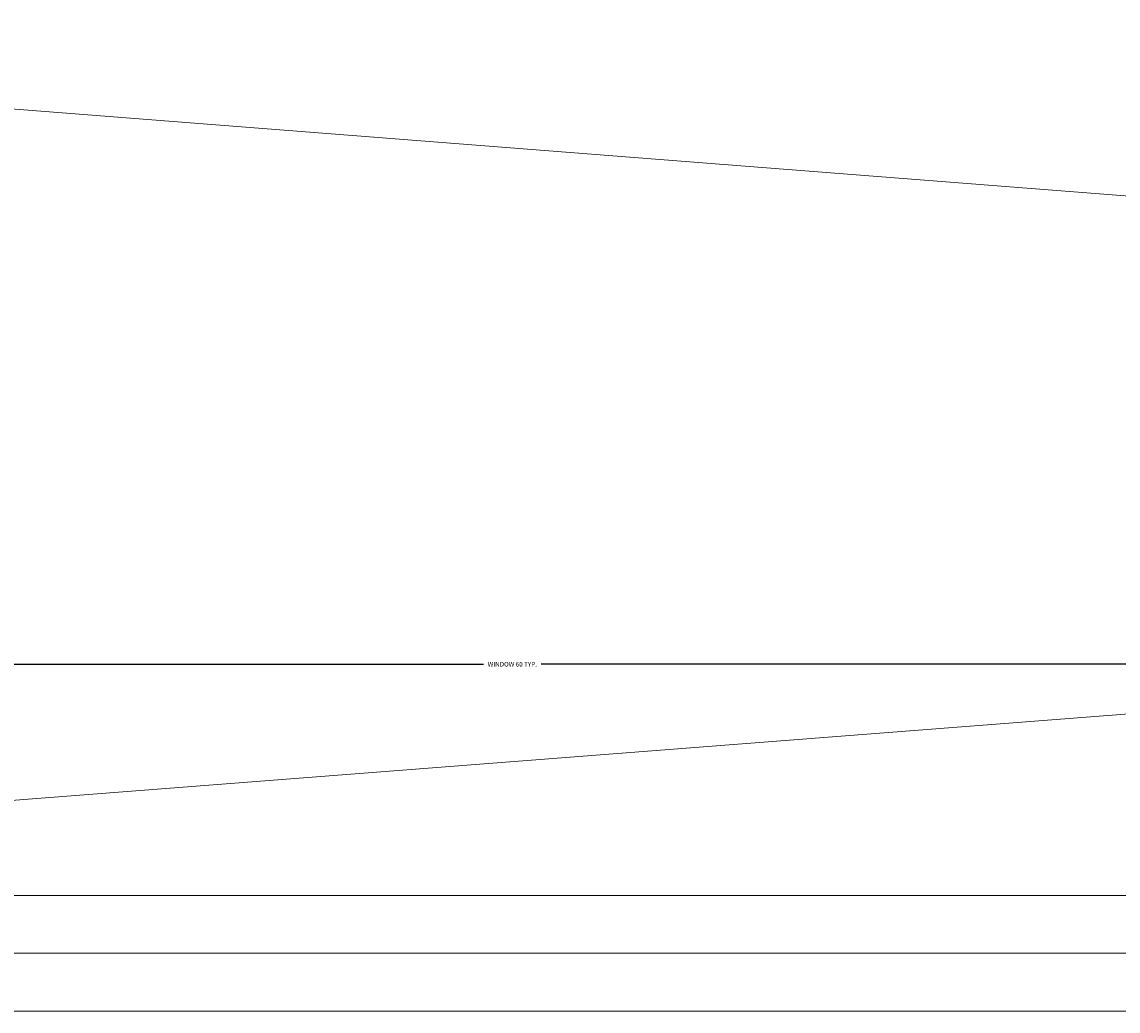
# Model space of a CAD drawing. Units: inches. Extents: x 1885 to 2748, y 783 to 2421.
# Tile 39 of 117: x 2056 to 2098, y 1520 to 1558. Entities that reach past the tile are written whole.
import ezdxf

# ---------------------------------------------------------------- set-up
doc = ezdxf.new("R2010")
doc.units = ezdxf.units.IN
for name, color, linetype, lineweight in [('A-ANNO-DIMS', 2, 'Continuous', 18), ('A-FLOR-OPEN', 8, 'Continuous', 13), ('A-GLAZ', 181, 'Continuous', 18)]:
    doc.layers.add(name, color=color, linetype=linetype, lineweight=lineweight)
doc.styles.get("Standard").update_dxf_attribs({"font": 'arial.ttf'})
doc.dimstyles.get("Standard").update_dxf_attribs({"dimtxt": 0.18, "dimasz": 0.18, "dimexe": 0.18, "dimexo": 0.0625, "dimgap": 0.09, "dimtad": 0, "dimtih": 1, "dimtoh": 1, "dimdec": 4, "dimzin": 0, "dimdsep": 46, "dimtxsty": 'Standard', "dimcen": 0.09, "dimadec": 0, "dimazin": 0, "dimtfac": 1, "dimtdec": 4, "dimtofl": 0, "dimtmove": 0, "dimatfit": 3, "dimfxl": 1, "dimtolj": 1, "dimtzin": 0, "dimarcsym": 0})

# ---------------------------------------------------------------- blocks, each defined once
blk = doc.blocks.new('WIN-60')
for p, q in [((0.004, 59.998), (4.504, 59.998)), ((0.004, 59.998), (0.004, -0.002)), ((4.504, 59.998), (2.254, 59.998)), ((2.254, 59.998), (2.254, -0.002)), ((4.504, -0.002), (4.504, 59.998)), ((2.254, -0.002), (0.004, -0.002)), ((0.004, -0.002), (4.504, -0.002))]:
    blk.add_line(p, q)
blk = doc.blocks.new('*D15')
at = {"layer": 'A-ANNO-DIMS', "color": 0, "lineweight": -2, "transparency": 16777216}
for p, q in [((2044.674, 1524.068), (2044.674, 1533.186)), ((2104.674, 1524.068), (2104.674, 1533.186)), ((2044.854, 1533.006), (2073.556, 1533.006)), ((2104.494, 1533.006), (2075.793, 1533.006))]:
    blk.add_line(p, q, dxfattribs=at)
at = {"layer": 'A-ANNO-DIMS', "color": 0, "transparency": 16777216}
for points in [[(2044.854, 1533.036), (2044.854, 1532.976), (2044.674, 1533.006)], [(2104.494, 1533.036), (2104.494, 1532.976), (2104.674, 1533.006)]]:
    blk.add_solid(points, dxfattribs=at)
at = {"layer": 'Defpoints', "color": 0, "transparency": 16777216}
for p in [(2104.674, 1533.006), (2044.674, 1524.006), (2104.674, 1524.006)]:
    blk.add_point(p, dxfattribs=at)
at = {"layer": 'A-ANNO-DIMS', "color": 0, "transparency": 16777216, "insert": (2074.674, 1533.006), "char_height": 0.18, "attachment_point": 5}
blk.add_mtext('\\A1;WINDOW 60 TYP.', dxfattribs=at)

msp = doc.modelspace()

# ---------------------------------------------------------------- linework, layer by layer
at = {"layer": 'A-FLOR-OPEN'}
for p, q in [((2007.274, 1524.006), (2447.274, 1558.006)), ((2447.274, 1524.006), (2011.774, 1558.006))]:
    msp.add_line(p, q, dxfattribs=at)

# ---------------------------------------------------------------- block references
at = {"layer": 'A-GLAZ', "extrusion": (0, 0, -1), "zscale": -1, "rotation": 90}
msp.add_blockref('WIN-60', (-2044.676, 1519.502), dxfattribs=at)

# ---------------------------------------------------------------- dimensions: what is measured, and where the dimension line sits
at = {"layer": 'A-ANNO-DIMS'}
dim = msp.add_linear_dim(base=(2104.674, 1533.006), p1=(2044.674, 1524.006), p2=(2104.674, 1524.006), text='WINDOW <> TYP.', dimstyle='Standard', override={"dimdec": 0, "dimlfac": 1, "dimrnd": 0, "dimzin": 0, "dimdsep": 46, "dimlunit": 2}, dxfattribs=at)
dim.commit()
dim.dimension.update_dxf_attribs({"geometry": '*D15', "text_midpoint": (2074.674, 1533.006)})

doc.saveas('drawing.dxf')
